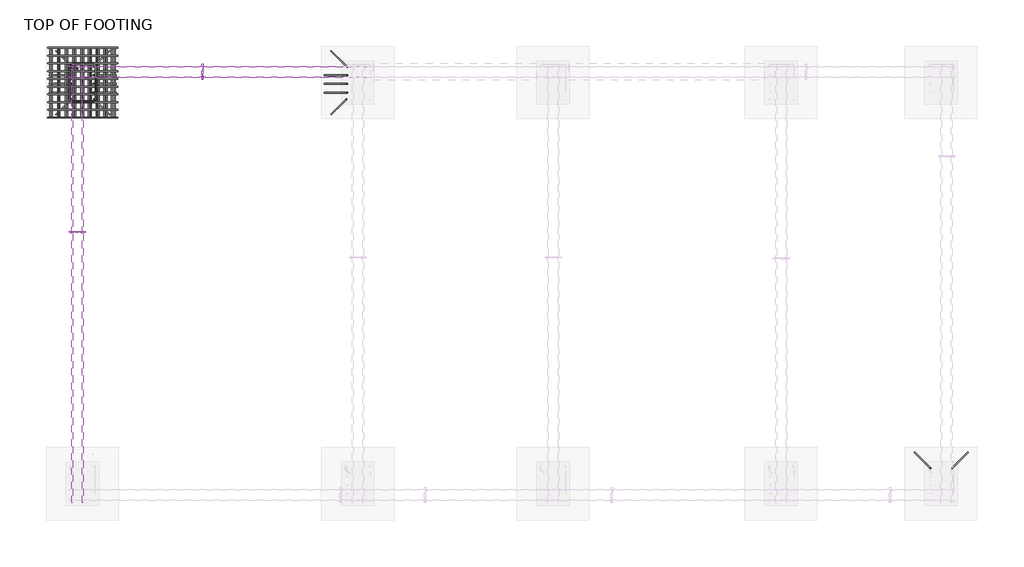
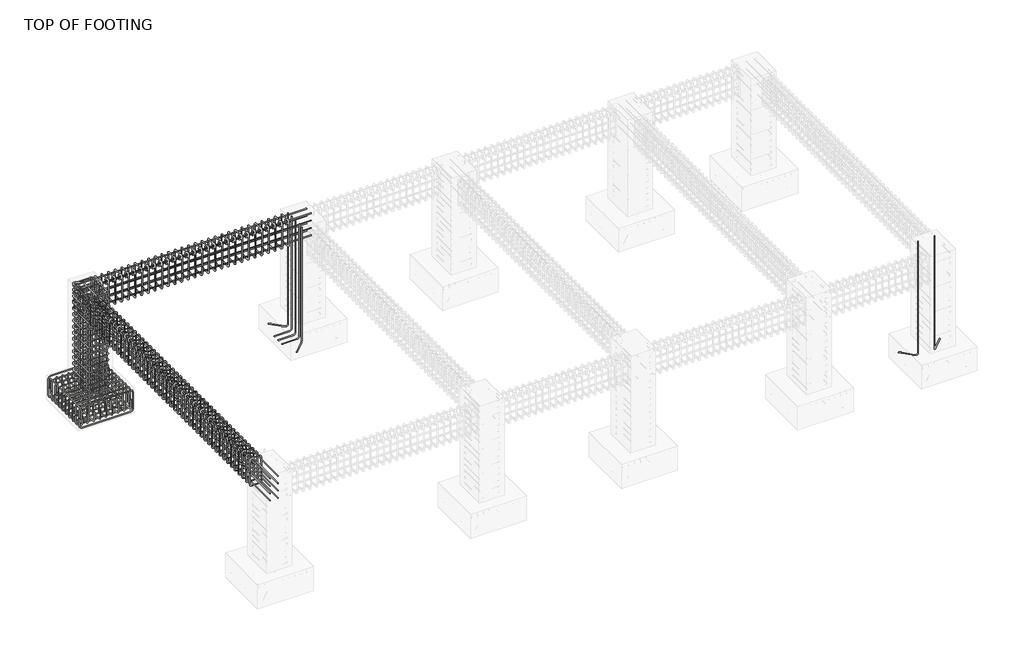
# One storey, part 5 of 9: 22 reinforcing bars.
"""IFC4 building model written with IfcOpenShell, lengths in millimetres."""

from ifc_helpers import new_model, si_unit, point, frame, origin, place, context, project, spatial, polyline, circle_curve, trimmed, segment, composite_curve, source, transform, mapped, element, save
from ifc_brep_helpers import swept_disk

model = new_model("IFC4")

# Units and contexts
model_context = context("Model", 3, world=origin())
ifc_project = project(units=[si_unit("LENGTHUNIT", "METRE", prefix="MILLI")], contexts=[model_context])

# Site, building, storey
site = spatial("IfcSite", under=ifc_project)
building = spatial("IfcBuilding", under=site)
storey = spatial("IfcBuildingStorey", under=building, Name="TOP OF FOOTING", Elevation=-1828.8)

# Reinforcing bars
placement = place(None, origin())
reinforcing_bar_shape = source(origin(), model_context, "Body", "SolidModel", [
    swept_disk(composite_curve([segment(polyline([(-11102.6174526, 4973.4875236, -2052.8356656), (-11102.6174526, 4973.4875236, -2200.1356656)]), True, "CONTINUOUS"), segment(trimmed(circle_curve(frame((-11148.9674526, 4973.4875236, -2200.1356656), z_axis=(0.0, 1.0, 0.0), x_axis=(46.350000000000364, 0.0, 0.0)), 46.35), [point((-11102.6174526, 4973.4875236, -2200.1356656))], [point((-11148.9674526, 4973.4875236, -2246.4856656))], True, "CARTESIAN"), True, "CONTINUOUS"), segment(polyline([(-11148.9674526, 4973.4875236, -2246.4856656), (-12017.5674526, 4973.4875236, -2246.4856656)]), True, "CONTINUOUS"), segment(trimmed(circle_curve(frame((-12017.5674526, 4973.4875236, -2200.1356656), z_axis=(0.0, 1.0, 0.0), x_axis=(0.0, 0.0, -46.350000000000364)), 46.35), [point((-12017.5674526, 4973.4875236, -2246.4856656))], [point((-12063.9174526, 4973.4875236, -2200.1356656))], True, "CARTESIAN"), True, "CONTINUOUS"), segment(polyline([(-12063.9174526, 4973.4875236, -2200.1356656), (-12063.9174526, 4973.4875236, -2052.8356656)]), True, "CONTINUOUS")], self_intersect=False), 6.35),
])
element("IfcReinforcingBar", 1, at=placement, inside=storey, context=model_context, shape_type="MappedRepresentation", body=[
    mapped(reinforcing_bar_shape, transform((0.0, 0.0, 0.0), x_axis=(1.0, 0.0, 0.0), y_axis=(0.0, 1.0, 0.0), z_axis=(0.0, 0.0, 1.0))),
    mapped(reinforcing_bar_shape, transform((0.0, -106.8111111, 0.0), x_axis=(1.0, 0.0, 0.0), y_axis=(0.0, 1.0, 0.0), z_axis=(0.0, 0.0, 1.0))),
    mapped(reinforcing_bar_shape, transform((0.0, -213.6222222, 0.0), x_axis=(1.0, 0.0, 0.0), y_axis=(0.0, 1.0, 0.0), z_axis=(0.0, 0.0, 1.0))),
    mapped(reinforcing_bar_shape, transform((0.0, -320.4333333, 0.0), x_axis=(1.0, 0.0, 0.0), y_axis=(0.0, 1.0, 0.0), z_axis=(0.0, 0.0, 1.0))),
    mapped(reinforcing_bar_shape, transform((0.0, -427.2444444, 0.0), x_axis=(1.0, 0.0, 0.0), y_axis=(0.0, 1.0, 0.0), z_axis=(0.0, 0.0, 1.0))),
    mapped(reinforcing_bar_shape, transform((0.0, -534.0555556, 0.0), x_axis=(1.0, 0.0, 0.0), y_axis=(0.0, 1.0, 0.0), z_axis=(0.0, 0.0, 1.0))),
    mapped(reinforcing_bar_shape, transform((0.0, -640.8666667, 0.0), x_axis=(1.0, 0.0, 0.0), y_axis=(0.0, 1.0, 0.0), z_axis=(0.0, 0.0, 1.0))),
    mapped(reinforcing_bar_shape, transform((0.0, -747.6777778, 0.0), x_axis=(1.0, 0.0, 0.0), y_axis=(0.0, 1.0, 0.0), z_axis=(0.0, 0.0, 1.0))),
    mapped(reinforcing_bar_shape, transform((0.0, -854.4888889, 0.0), x_axis=(1.0, 0.0, 0.0), y_axis=(0.0, 1.0, 0.0), z_axis=(0.0, 0.0, 1.0))),
    mapped(reinforcing_bar_shape, transform((0.0, -961.3, 0.0), x_axis=(1.0, 0.0, 0.0), y_axis=(0.0, 1.0, 0.0), z_axis=(0.0, 0.0, 1.0))),
])
reinforcing_bar_2_shape = source(origin(), model_context, "Body", "SolidModel", [
    swept_disk(composite_curve([segment(polyline([(-12063.9174526, 4973.4875236, -2041.8), (-12063.9174526, 4973.4875236, -1894.5)]), True, "CONTINUOUS"), segment(trimmed(circle_curve(frame((-12017.5674526, 4973.4875236, -1894.5), z_axis=(0.0, 1.0, 0.0), x_axis=(-46.350000000000364, 0.0, 0.0)), 46.35), [point((-12063.9174526, 4973.4875236, -1894.5))], [point((-12017.5674526, 4973.4875236, -1848.15))], True, "CARTESIAN"), True, "CONTINUOUS"), segment(polyline([(-12017.5674526, 4973.4875236, -1848.15), (-11148.9674526, 4973.4875236, -1848.15)]), True, "CONTINUOUS"), segment(trimmed(circle_curve(frame((-11148.9674526, 4973.4875236, -1894.5), z_axis=(0.0, 1.0, 0.0), x_axis=(0.0, 0.0, 46.34999999999991)), 46.35), [point((-11148.9674526, 4973.4875236, -1848.15))], [point((-11102.6174526, 4973.4875236, -1894.5))], True, "CARTESIAN"), True, "CONTINUOUS"), segment(polyline([(-11102.6174526, 4973.4875236, -1894.5), (-11102.6174526, 4973.4875236, -2041.8)]), True, "CONTINUOUS")], self_intersect=False), 6.35),
])
element("IfcReinforcingBar", 2, at=placement, inside=storey, context=model_context, shape_type="MappedRepresentation", body=[
    mapped(reinforcing_bar_2_shape, transform((0.0, 0.0, 0.0), x_axis=(1.0, 0.0, 0.0), y_axis=(0.0, 1.0, 0.0), z_axis=(0.0, 0.0, 1.0))),
    mapped(reinforcing_bar_2_shape, transform((0.0, -106.8111111, 0.0), x_axis=(1.0, 0.0, 0.0), y_axis=(0.0, 1.0, 0.0), z_axis=(0.0, 0.0, 1.0))),
    mapped(reinforcing_bar_2_shape, transform((0.0, -213.6222222, 0.0), x_axis=(1.0, 0.0, 0.0), y_axis=(0.0, 1.0, 0.0), z_axis=(0.0, 0.0, 1.0))),
    mapped(reinforcing_bar_2_shape, transform((0.0, -320.4333333, 0.0), x_axis=(1.0, 0.0, 0.0), y_axis=(0.0, 1.0, 0.0), z_axis=(0.0, 0.0, 1.0))),
    mapped(reinforcing_bar_2_shape, transform((0.0, -427.2444444, 0.0), x_axis=(1.0, 0.0, 0.0), y_axis=(0.0, 1.0, 0.0), z_axis=(0.0, 0.0, 1.0))),
    mapped(reinforcing_bar_2_shape, transform((0.0, -534.0555556, 0.0), x_axis=(1.0, 0.0, 0.0), y_axis=(0.0, 1.0, 0.0), z_axis=(0.0, 0.0, 1.0))),
    mapped(reinforcing_bar_2_shape, transform((0.0, -640.8666667, 0.0), x_axis=(1.0, 0.0, 0.0), y_axis=(0.0, 1.0, 0.0), z_axis=(0.0, 0.0, 1.0))),
    mapped(reinforcing_bar_2_shape, transform((0.0, -747.6777778, 0.0), x_axis=(1.0, 0.0, 0.0), y_axis=(0.0, 1.0, 0.0), z_axis=(0.0, 0.0, 1.0))),
    mapped(reinforcing_bar_2_shape, transform((0.0, -854.4888889, 0.0), x_axis=(1.0, 0.0, 0.0), y_axis=(0.0, 1.0, 0.0), z_axis=(0.0, 0.0, 1.0))),
    mapped(reinforcing_bar_2_shape, transform((0.0, -961.3, 0.0), x_axis=(1.0, 0.0, 0.0), y_axis=(0.0, 1.0, 0.0), z_axis=(0.0, 0.0, 1.0))),
])
reinforcing_bar_3_shape = source(origin(), model_context, "Body", "SolidModel", [
    swept_disk(composite_curve([segment(polyline([(-12013.2674526, 4973.4875236, -2020.15), (-12013.2674526, 4973.4875236, -2167.45)]), True, "CONTINUOUS"), segment(trimmed(circle_curve(frame((-12013.2674526, 4927.1375236, -2167.45), z_axis=(-1.0, 0.0, 0.0), x_axis=(0.0, 46.349999999999454, 0.0)), 46.35), [point((-12013.2674526, 4973.4875236, -2167.45))], [point((-12013.2674526, 4927.1375236, -2213.8))], True, "CARTESIAN"), True, "CONTINUOUS"), segment(polyline([(-12013.2674526, 4927.1375236, -2213.8), (-12013.2674526, 4058.5375236, -2213.8)]), True, "CONTINUOUS"), segment(trimmed(circle_curve(frame((-12013.2674526, 4058.5375236, -2167.45), z_axis=(-1.0, 0.0, 0.0), x_axis=(0.0, 0.0, -46.350000000000364)), 46.35), [point((-12013.2674526, 4058.5375236, -2213.8))], [point((-12013.2674526, 4012.1875236, -2167.45))], True, "CARTESIAN"), True, "CONTINUOUS"), segment(polyline([(-12013.2674526, 4012.1875236, -2167.45), (-12013.2674526, 4012.1875236, -2020.15)]), True, "CONTINUOUS")], self_intersect=False), 6.35),
])
element("IfcReinforcingBar", 3, at=placement, inside=storey, context=model_context, shape_type="MappedRepresentation", body=[
    mapped(reinforcing_bar_3_shape, transform((0.0, 0.0, 0.0), x_axis=(1.0, 0.0, 0.0), y_axis=(0.0, 1.0, 0.0), z_axis=(0.0, 0.0, 1.0))),
    mapped(reinforcing_bar_3_shape, transform((108.8370374, 0.0, 0.0), x_axis=(1.0, 0.0, 0.0), y_axis=(0.0, 1.0, 0.0), z_axis=(0.0, 0.0, 1.0))),
    mapped(reinforcing_bar_3_shape, transform((217.6740748, 0.0, 0.0), x_axis=(1.0, 0.0, 0.0), y_axis=(0.0, 1.0, 0.0), z_axis=(0.0, 0.0, 1.0))),
    mapped(reinforcing_bar_3_shape, transform((326.5111123, 0.0, 0.0), x_axis=(1.0, 0.0, 0.0), y_axis=(0.0, 1.0, 0.0), z_axis=(0.0, 0.0, 1.0))),
    mapped(reinforcing_bar_3_shape, transform((435.3481497, 0.0, 0.0), x_axis=(1.0, 0.0, 0.0), y_axis=(0.0, 1.0, 0.0), z_axis=(0.0, 0.0, 1.0))),
    mapped(reinforcing_bar_3_shape, transform((544.1851871, 0.0, 0.0), x_axis=(1.0, 0.0, 0.0), y_axis=(0.0, 1.0, 0.0), z_axis=(0.0, 0.0, 1.0))),
    mapped(reinforcing_bar_3_shape, transform((653.0222245, 0.0, 0.0), x_axis=(1.0, 0.0, 0.0), y_axis=(0.0, 1.0, 0.0), z_axis=(0.0, 0.0, 1.0))),
    mapped(reinforcing_bar_3_shape, transform((761.8592619, 0.0, 0.0), x_axis=(1.0, 0.0, 0.0), y_axis=(0.0, 1.0, 0.0), z_axis=(0.0, 0.0, 1.0))),
    mapped(reinforcing_bar_3_shape, transform((870.6962994, 0.0, 0.0), x_axis=(1.0, 0.0, 0.0), y_axis=(0.0, 1.0, 0.0), z_axis=(0.0, 0.0, 1.0))),
])
reinforcing_bar_4_shape = source(origin(), model_context, "Body", "SolidModel", [
    swept_disk(composite_curve([segment(polyline([(-11180.7455787, 4973.4875236, -2076.9782245), (-11180.7455787, 4973.4875236, -1929.6782245)]), True, "CONTINUOUS"), segment(trimmed(circle_curve(frame((-11180.7455787, 4927.1375236, -1929.6782245), z_axis=(1.0, 0.0, 0.0), x_axis=(0.0, 46.349999999999454, 0.0)), 46.35), [point((-11180.7455787, 4973.4875236, -1929.6782245))], [point((-11180.7455787, 4927.1375236, -1883.3282245))], True, "CARTESIAN"), True, "CONTINUOUS"), segment(polyline([(-11180.7455787, 4927.1375236, -1883.3282245), (-11180.7455787, 4058.5375236, -1883.3282245)]), True, "CONTINUOUS"), segment(trimmed(circle_curve(frame((-11180.7455787, 4058.5375236, -1929.6782245), z_axis=(1.0, 0.0, 0.0), x_axis=(0.0, 0.0, 46.34999999999991)), 46.35), [point((-11180.7455787, 4058.5375236, -1883.3282245))], [point((-11180.7455787, 4012.1875236, -1929.6782245))], True, "CARTESIAN"), True, "CONTINUOUS"), segment(polyline([(-11180.7455787, 4012.1875236, -1929.6782245), (-11180.7455787, 4012.1875236, -2076.9782245)]), True, "CONTINUOUS")], self_intersect=False), 6.35),
])
element("IfcReinforcingBar", 4, at=placement, inside=storey, context=model_context, shape_type="MappedRepresentation", body=[
    mapped(reinforcing_bar_4_shape, transform((0.0, 0.0, 0.0), x_axis=(1.0, 0.0, 0.0), y_axis=(0.0, 1.0, 0.0), z_axis=(0.0, 0.0, 1.0))),
    mapped(reinforcing_bar_4_shape, transform((-106.3275638, 0.0, 0.0), x_axis=(1.0, 0.0, 0.0), y_axis=(0.0, 1.0, 0.0), z_axis=(0.0, 0.0, 1.0))),
    mapped(reinforcing_bar_4_shape, transform((-212.6551275, 0.0, 0.0), x_axis=(1.0, 0.0, 0.0), y_axis=(0.0, 1.0, 0.0), z_axis=(0.0, 0.0, 1.0))),
    mapped(reinforcing_bar_4_shape, transform((-318.9826913, 0.0, 0.0), x_axis=(1.0, 0.0, 0.0), y_axis=(0.0, 1.0, 0.0), z_axis=(0.0, 0.0, 1.0))),
    mapped(reinforcing_bar_4_shape, transform((-425.310255, 0.0, 0.0), x_axis=(1.0, 0.0, 0.0), y_axis=(0.0, 1.0, 0.0), z_axis=(0.0, 0.0, 1.0))),
    mapped(reinforcing_bar_4_shape, transform((-531.6378188, 0.0, 0.0), x_axis=(1.0, 0.0, 0.0), y_axis=(0.0, 1.0, 0.0), z_axis=(0.0, 0.0, 1.0))),
    mapped(reinforcing_bar_4_shape, transform((-637.9653825, 0.0, 0.0), x_axis=(1.0, 0.0, 0.0), y_axis=(0.0, 1.0, 0.0), z_axis=(0.0, 0.0, 1.0))),
    mapped(reinforcing_bar_4_shape, transform((-744.2929463, 0.0, 0.0), x_axis=(1.0, 0.0, 0.0), y_axis=(0.0, 1.0, 0.0), z_axis=(0.0, 0.0, 1.0))),
    mapped(reinforcing_bar_4_shape, transform((-850.62051, 0.0, 0.0), x_axis=(1.0, 0.0, 0.0), y_axis=(0.0, 1.0, 0.0), z_axis=(0.0, 0.0, 1.0))),
])
reinforcing_bar_5_shape = source(origin(), model_context, "Body", "SolidModel", [
    swept_disk(composite_curve([segment(polyline([(-11730.5674526, 4357.3343029, -40.0), (-11730.5674526, 4357.3343029, -2148.1729582)]), True, "CONTINUOUS"), segment(trimmed(circle_curve(frame((-11776.9174526, 4357.3343029, -2148.1729582), z_axis=(0.0, 1.0, 0.0), x_axis=(46.350000000000364, 0.0, 0.0)), 46.35), [point((-11730.5674526, 4357.3343029, -2148.1729582))], [point((-11776.9174526, 4357.3343029, -2194.5229582))], True, "CARTESIAN"), True, "CONTINUOUS"), segment(polyline([(-11776.9174526, 4357.3343029, -2194.5229582), (-12043.513478, 4357.3343029, -2194.5229582)]), True, "CONTINUOUS")], self_intersect=False), 6.35),
])
element("IfcReinforcingBar", 5, at=placement, inside=storey, context=model_context, shape_type="MappedRepresentation", body=[
    mapped(reinforcing_bar_5_shape, transform((0.0, 0.0, 0.0), x_axis=(1.0, 0.0, 0.0), y_axis=(0.0, 1.0, 0.0), z_axis=(0.0, 0.0, 1.0))),
    mapped(reinforcing_bar_5_shape, transform((0.0, 119.1364467, 0.0), x_axis=(1.0, 0.0, 0.0), y_axis=(0.0, 1.0, 0.0), z_axis=(0.0, 0.0, 1.0))),
    mapped(reinforcing_bar_5_shape, transform((0.0, 238.2728934, 0.0), x_axis=(1.0, 0.0, 0.0), y_axis=(0.0, 1.0, 0.0), z_axis=(0.0, 0.0, 1.0))),
])
reinforcing_bar_6_shape = source(origin(), model_context, "Body", "SolidModel", [
    swept_disk(composite_curve([segment(polyline([(-11652.6560921, 4681.5617582, -1782.45), (-11708.399655, 4737.3053212, -1782.45)]), True, "CONTINUOUS"), segment(trimmed(circle_curve(frame((-11730.5674526, 4715.1375236, -1782.45), z_axis=(0.0, 0.0, 1.0), x_axis=(22.167797600000995, 22.167797600000085, 0.0)), 31.35), [point((-11708.399655, 4737.3053212, -1782.45))], [point((-11761.9174526, 4715.1375236, -1782.45))], True, "CARTESIAN"), True, "CONTINUOUS"), segment(polyline([(-11761.9174526, 4715.1375236, -1782.45), (-11761.9174526, 4270.5375236, -1782.45)]), True, "CONTINUOUS"), segment(trimmed(circle_curve(frame((-11730.5674526, 4270.5375236, -1782.45), z_axis=(0.0, 0.0, 1.0), x_axis=(-31.350000000000364, 0.0, 0.0)), 31.35), [point((-11761.9174526, 4270.5375236, -1782.45))], [point((-11730.5674526, 4239.1875236, -1782.45))], True, "CARTESIAN"), True, "CONTINUOUS"), segment(polyline([(-11730.5674526, 4239.1875236, -1782.45), (-11435.9674526, 4239.1875236, -1782.45)]), True, "CONTINUOUS"), segment(trimmed(circle_curve(frame((-11435.9674526, 4270.5277043, -1783.2345856), z_axis=(0.0, 0.025026655153786315, 0.9996867842138424), x_axis=(0.0, -31.34018070000002, 0.7845855999999003)), 31.35), [point((-11435.9674526, 4239.1875236, -1782.45))], [point((-11404.6174526, 4270.5277043, -1783.2345856))], True, "CARTESIAN"), True, "CONTINUOUS"), segment(polyline([(-11404.6174526, 4270.5277043, -1783.2345856), (-11404.6174526, 4715.1473429, -1794.3654144)]), True, "CONTINUOUS"), segment(trimmed(circle_curve(frame((-11435.9674526, 4715.1473429, -1794.3654144), z_axis=(0.0, 0.025026655153786315, 0.9996867842138424), x_axis=(31.350000000000364, 0.0, 0.0)), 31.35), [point((-11404.6174526, 4715.1473429, -1794.3654144))], [point((-11435.9674526, 4746.4875236, -1795.15))], True, "CARTESIAN"), True, "CONTINUOUS"), segment(polyline([(-11435.9674526, 4746.4875236, -1795.15), (-11730.5674526, 4746.4875236, -1795.15)]), True, "CONTINUOUS"), segment(trimmed(circle_curve(frame((-11730.5674526, 4715.1375236, -1795.15), z_axis=(0.0, 0.0, 1.0), x_axis=(0.0, 31.349999999999454, 0.0)), 31.35), [point((-11730.5674526, 4746.4875236, -1795.15))], [point((-11752.7352502, 4692.969726, -1795.15))], True, "CARTESIAN"), True, "CONTINUOUS"), segment(polyline([(-11752.7352502, 4692.969726, -1795.15), (-11696.9916873, 4637.226163, -1795.15)]), True, "CONTINUOUS")], self_intersect=False), 6.35),
])
element("IfcReinforcingBar", 6, at=placement, inside=storey, context=model_context, shape_type="MappedRepresentation", body=[
    mapped(reinforcing_bar_6_shape, transform((0.0, 0.0, 0.0), x_axis=(1.0, 0.0, 0.0), y_axis=(0.0, 1.0, 0.0), z_axis=(0.0, 0.0, 1.0))),
    mapped(reinforcing_bar_6_shape, transform((0.0, 0.0, 115.74), x_axis=(1.0, 0.0, 0.0), y_axis=(0.0, 1.0, 0.0), z_axis=(0.0, 0.0, 1.0))),
    mapped(reinforcing_bar_6_shape, transform((0.0, 0.0, 231.48), x_axis=(1.0, 0.0, 0.0), y_axis=(0.0, 1.0, 0.0), z_axis=(0.0, 0.0, 1.0))),
    mapped(reinforcing_bar_6_shape, transform((0.0, 0.0, 347.22), x_axis=(1.0, 0.0, 0.0), y_axis=(0.0, 1.0, 0.0), z_axis=(0.0, 0.0, 1.0))),
    mapped(reinforcing_bar_6_shape, transform((0.0, 0.0, 462.96), x_axis=(1.0, 0.0, 0.0), y_axis=(0.0, 1.0, 0.0), z_axis=(0.0, 0.0, 1.0))),
    mapped(reinforcing_bar_6_shape, transform((0.0, 0.0, 578.7), x_axis=(1.0, 0.0, 0.0), y_axis=(0.0, 1.0, 0.0), z_axis=(0.0, 0.0, 1.0))),
    mapped(reinforcing_bar_6_shape, transform((0.0, 0.0, 694.44), x_axis=(1.0, 0.0, 0.0), y_axis=(0.0, 1.0, 0.0), z_axis=(0.0, 0.0, 1.0))),
    mapped(reinforcing_bar_6_shape, transform((0.0, 0.0, 810.18), x_axis=(1.0, 0.0, 0.0), y_axis=(0.0, 1.0, 0.0), z_axis=(0.0, 0.0, 1.0))),
    mapped(reinforcing_bar_6_shape, transform((0.0, 0.0, 925.92), x_axis=(1.0, 0.0, 0.0), y_axis=(0.0, 1.0, 0.0), z_axis=(0.0, 0.0, 1.0))),
    mapped(reinforcing_bar_6_shape, transform((0.0, 0.0, 1041.66), x_axis=(1.0, 0.0, 0.0), y_axis=(0.0, 1.0, 0.0), z_axis=(0.0, 0.0, 1.0))),
    mapped(reinforcing_bar_6_shape, transform((0.0, 0.0, 1157.4), x_axis=(1.0, 0.0, 0.0), y_axis=(0.0, 1.0, 0.0), z_axis=(0.0, 0.0, 1.0))),
    mapped(reinforcing_bar_6_shape, transform((0.0, 0.0, 1273.14), x_axis=(1.0, 0.0, 0.0), y_axis=(0.0, 1.0, 0.0), z_axis=(0.0, 0.0, 1.0))),
    mapped(reinforcing_bar_6_shape, transform((0.0, 0.0, 1388.88), x_axis=(1.0, 0.0, 0.0), y_axis=(0.0, 1.0, 0.0), z_axis=(0.0, 0.0, 1.0))),
    mapped(reinforcing_bar_6_shape, transform((0.0, 0.0, 1504.62), x_axis=(1.0, 0.0, 0.0), y_axis=(0.0, 1.0, 0.0), z_axis=(0.0, 0.0, 1.0))),
    mapped(reinforcing_bar_6_shape, transform((0.0, 0.0, 1620.36), x_axis=(1.0, 0.0, 0.0), y_axis=(0.0, 1.0, 0.0), z_axis=(0.0, 0.0, 1.0))),
    mapped(reinforcing_bar_6_shape, transform((0.0, 0.0, 1736.1), x_axis=(1.0, 0.0, 0.0), y_axis=(0.0, 1.0, 0.0), z_axis=(0.0, 0.0, 1.0))),
])
element("IfcReinforcingBar", 7, at=placement, inside=storey, context=model_context, shape_type="SolidModel", body=[
    swept_disk(composite_curve([segment(polyline([(-11730.5674526, 4712.2713987, -40.0), (-11730.5674526, 4712.2713987, -2148.1729582)]), True, "CONTINUOUS"), segment(trimmed(circle_curve(frame((-11763.3418519, 4745.045798, -2148.1729582), z_axis=(0.7071067811865507, 0.7071067811865444, 0.0), x_axis=(32.77439930000037, -32.77439930000037, 0.0)), 46.35), [point((-11730.5674526, 4712.2713987, -2148.1729582))], [point((-11763.3418519, 4745.045798, -2194.5229582))], True, "CARTESIAN"), True, "CONTINUOUS"), segment(polyline([(-11763.3418519, 4745.045798, -2194.5229582), (-11951.8537093, 4933.5576554, -2194.5229582)]), True, "CONTINUOUS")], self_intersect=False), 6.35),
])
element("IfcReinforcingBar", 8, at=placement, inside=storey, context=model_context, shape_type="SolidModel", body=[
    swept_disk(composite_curve([segment(polyline([(-11740.5132324, 4263.4578687, -40.0), (-11740.5132324, 4263.4578687, -2148.1729582)]), True, "CONTINUOUS"), segment(trimmed(circle_curve(frame((-11773.2876317, 4230.6834694, -2148.1729582), z_axis=(-0.707106781186547, 0.707106781186548, 0.0), x_axis=(32.77439929999855, 32.77439930000037, 0.0)), 46.35), [point((-11740.5132324, 4263.4578687, -2148.1729582))], [point((-11773.2876317, 4230.6834694, -2194.5229582))], True, "CARTESIAN"), True, "CONTINUOUS"), segment(polyline([(-11773.2876317, 4230.6834694, -2194.5229582), (-11951.8537093, 4052.1173918, -2194.5229582)]), True, "CONTINUOUS")], self_intersect=False), 6.35),
])
element("IfcReinforcingBar", 9, at=placement, inside=storey, context=model_context, shape_type="SolidModel", body=[
    swept_disk(composite_curve([segment(polyline([(-11435.9674526, 4712.2713987, -40.0), (-11435.9674526, 4712.2713987, -2148.1729582)]), True, "CONTINUOUS"), segment(trimmed(circle_curve(frame((-11403.1930533, 4745.045798, -2148.1729582), z_axis=(0.7071067811865507, -0.7071067811865444, 0.0), x_axis=(-32.77439930000037, -32.77439930000037, 0.0)), 46.35), [point((-11435.9674526, 4712.2713987, -2148.1729582))], [point((-11403.1930533, 4745.045798, -2194.5229582))], True, "CARTESIAN"), True, "CONTINUOUS"), segment(polyline([(-11403.1930533, 4745.045798, -2194.5229582), (-11214.6811959, 4933.5576554, -2194.5229582)]), True, "CONTINUOUS")], self_intersect=False), 6.35),
])
element("IfcReinforcingBar", 10, at=placement, inside=storey, context=model_context, shape_type="SolidModel", body=[
    swept_disk(composite_curve([segment(polyline([(-11426.0216728, 4263.4578687, -40.0), (-11426.0216728, 4263.4578687, -2148.1729582)]), True, "CONTINUOUS"), segment(trimmed(circle_curve(frame((-11393.2472735, 4230.6834694, -2148.1729582), z_axis=(-0.707106781186547, -0.707106781186548, 0.0), x_axis=(-32.77439930000037, 32.77439930000037, 0.0)), 46.35), [point((-11426.0216728, 4263.4578687, -2148.1729582))], [point((-11393.2472735, 4230.6834694, -2194.5229582))], True, "CARTESIAN"), True, "CONTINUOUS"), segment(polyline([(-11393.2472735, 4230.6834694, -2194.5229582), (-11214.6811959, 4052.1173918, -2194.5229582)]), True, "CONTINUOUS")], self_intersect=False), 6.35),
])
reinforcing_bar_7_shape = source(origin(), model_context, "Body", "SolidModel", [
    swept_disk(composite_curve([segment(polyline([(-11435.9674526, 4357.3343029, -40.0), (-11435.9674526, 4357.3343029, -2148.1729582)]), True, "CONTINUOUS"), segment(trimmed(circle_curve(frame((-11389.6174526, 4357.3343029, -2148.1729582), z_axis=(0.0, -1.0, 0.0), x_axis=(-46.350000000000364, 0.0, 0.0)), 46.35), [point((-11435.9674526, 4357.3343029, -2148.1729582))], [point((-11389.6174526, 4357.3343029, -2194.5229582))], True, "CARTESIAN"), True, "CONTINUOUS"), segment(polyline([(-11389.6174526, 4357.3343029, -2194.5229582), (-11123.0214272, 4357.3343029, -2194.5229582)]), True, "CONTINUOUS")], self_intersect=False), 6.35),
])
element("IfcReinforcingBar", 11, at=placement, inside=storey, context=model_context, shape_type="MappedRepresentation", body=[
    mapped(reinforcing_bar_7_shape, transform((0.0, 0.0, 0.0), x_axis=(1.0, 0.0, 0.0), y_axis=(0.0, 1.0, 0.0), z_axis=(0.0, 0.0, 1.0))),
    mapped(reinforcing_bar_7_shape, transform((0.0, 119.1364467, 0.0), x_axis=(1.0, 0.0, 0.0), y_axis=(0.0, 1.0, 0.0), z_axis=(0.0, 0.0, 1.0))),
    mapped(reinforcing_bar_7_shape, transform((0.0, 238.2728934, 0.0), x_axis=(1.0, 0.0, 0.0), y_axis=(0.0, 1.0, 0.0), z_axis=(0.0, 0.0, 1.0))),
])
reinforcing_bar_8_shape = source(origin(), model_context, "Body", "SolidModel", [
    swept_disk(composite_curve([segment(polyline([(-7930.5674526, 4357.3343029, -40.0), (-7930.5674526, 4357.3343029, -2148.1729582)]), True, "CONTINUOUS"), segment(trimmed(circle_curve(frame((-7976.9174526, 4357.3343029, -2148.1729582), z_axis=(0.0, 1.0, 0.0), x_axis=(46.349999999999454, 0.0, 0.0)), 46.35), [point((-7930.5674526, 4357.3343029, -2148.1729582))], [point((-7976.9174526, 4357.3343029, -2194.5229582))], True, "CARTESIAN"), True, "CONTINUOUS"), segment(polyline([(-7976.9174526, 4357.3343029, -2194.5229582), (-8243.513478, 4357.3343029, -2194.5229582)]), True, "CONTINUOUS")], self_intersect=False), 6.35),
])
element("IfcReinforcingBar", 12, at=placement, inside=storey, context=model_context, shape_type="MappedRepresentation", body=[
    mapped(reinforcing_bar_8_shape, transform((0.0, 0.0, 0.0), x_axis=(1.0, 0.0, 0.0), y_axis=(0.0, 1.0, 0.0), z_axis=(0.0, 0.0, 1.0))),
    mapped(reinforcing_bar_8_shape, transform((0.0, 119.1364467, 0.0), x_axis=(1.0, 0.0, 0.0), y_axis=(0.0, 1.0, 0.0), z_axis=(0.0, 0.0, 1.0))),
    mapped(reinforcing_bar_8_shape, transform((0.0, 238.2728934, 0.0), x_axis=(1.0, 0.0, 0.0), y_axis=(0.0, 1.0, 0.0), z_axis=(0.0, 0.0, 1.0))),
])
element("IfcReinforcingBar", 13, at=placement, inside=storey, context=model_context, shape_type="SolidModel", body=[
    swept_disk(composite_curve([segment(polyline([(-7930.5674526, 4712.2713987, -40.0), (-7930.5674526, 4712.2713987, -2148.1729582)]), True, "CONTINUOUS"), segment(trimmed(circle_curve(frame((-7963.3418519, 4745.045798, -2148.1729582), z_axis=(0.7071067811865507, 0.7071067811865444, 0.0), x_axis=(32.77439929999946, -32.77439930000037, 0.0)), 46.35), [point((-7930.5674526, 4712.2713987, -2148.1729582))], [point((-7963.3418519, 4745.045798, -2194.5229582))], True, "CARTESIAN"), True, "CONTINUOUS"), segment(polyline([(-7963.3418519, 4745.045798, -2194.5229582), (-8151.8537093, 4933.5576554, -2194.5229582)]), True, "CONTINUOUS")], self_intersect=False), 6.35),
])
element("IfcReinforcingBar", 14, at=placement, inside=storey, context=model_context, shape_type="SolidModel", body=[
    swept_disk(composite_curve([segment(polyline([(-7940.5132324, 4263.4578687, -40.0), (-7940.5132324, 4263.4578687, -2148.1729582)]), True, "CONTINUOUS"), segment(trimmed(circle_curve(frame((-7973.2876317, 4230.6834694, -2148.1729582), z_axis=(-0.707106781186547, 0.707106781186548, 0.0), x_axis=(32.77439930000037, 32.77439930000037, 0.0)), 46.35), [point((-7940.5132324, 4263.4578687, -2148.1729582))], [point((-7973.2876317, 4230.6834694, -2194.5229582))], True, "CARTESIAN"), True, "CONTINUOUS"), segment(polyline([(-7973.2876317, 4230.6834694, -2194.5229582), (-8151.8537093, 4052.1173918, -2194.5229582)]), True, "CONTINUOUS")], self_intersect=False), 6.35),
])
element("IfcReinforcingBar", 15, at=placement, inside=storey, context=model_context, shape_type="SolidModel", body=[
    swept_disk(composite_curve([segment(polyline([(129.4325474, -832.8986176, -40.0), (129.4325474, -832.8986176, -2148.1729582)]), True, "CONTINUOUS"), segment(trimmed(circle_curve(frame((96.6581481, -800.1242183, -2148.1729582), z_axis=(0.7071067811865507, 0.7071067811865444, 0.0), x_axis=(32.7743993, -32.774399299999914, 0.0)), 46.35), [point((129.4325474, -832.8986176, -2148.1729582))], [point((96.6581481, -800.1242183, -2194.5229582))], True, "CARTESIAN"), True, "CONTINUOUS"), segment(polyline([(96.6581481, -800.1242183, -2194.5229582), (-91.8537093, -611.6123609, -2194.5229582)]), True, "CONTINUOUS")], self_intersect=False), 6.35),
])
element("IfcReinforcingBar", 16, at=placement, inside=storey, context=model_context, shape_type="SolidModel", body=[
    swept_disk(composite_curve([segment(polyline([(424.0325474, -832.8986176, -40.0), (424.0325474, -832.8986176, -2148.1729582)]), True, "CONTINUOUS"), segment(trimmed(circle_curve(frame((456.8069467, -800.1242183, -2148.1729582), z_axis=(0.7071067811865507, -0.7071067811865444, 0.0), x_axis=(-32.77439930000003, -32.774399299999914, 0.0)), 46.35), [point((424.0325474, -832.8986176, -2148.1729582))], [point((456.8069467, -800.1242183, -2194.5229582))], True, "CARTESIAN"), True, "CONTINUOUS"), segment(polyline([(456.8069467, -800.1242183, -2194.5229582), (645.3188041, -611.6123609, -2194.5229582)]), True, "CONTINUOUS")], self_intersect=False), 6.35),
])
reinforcing_bar_9_shape = source(origin(), model_context, "Body", "SolidModel", [
    swept_disk(composite_curve([segment(polyline([(-11652.6560921, 4186.4875236, -111.2757654), (-11708.399655, 4186.4875236, -55.5322024)]), True, "CONTINUOUS"), segment(trimmed(circle_curve(frame((-11730.5674526, 4186.4875236, -77.7), z_axis=(0.0, -1.0, 0.0), x_axis=(22.167797600000995, 0.0, 22.1677976)), 31.35), [point((-11708.399655, 4186.4875236, -55.5322024))], [point((-11761.9174526, 4186.4875236, -77.7))], True, "CARTESIAN"), True, "CONTINUOUS"), segment(polyline([(-11761.9174526, 4186.4875236, -77.7), (-11761.9174526, 4186.4875236, -522.3)]), True, "CONTINUOUS"), segment(trimmed(circle_curve(frame((-11730.5674526, 4186.4875236, -522.3), z_axis=(0.0, -1.0, 0.0), x_axis=(-31.350000000000364, 0.0, 0.0)), 31.35), [point((-11761.9174526, 4186.4875236, -522.3))], [point((-11730.5674526, 4186.4875236, -553.65))], True, "CARTESIAN"), True, "CONTINUOUS"), segment(polyline([(-11730.5674526, 4186.4875236, -553.65), (-11585.9674526, 4186.4875236, -553.65)]), True, "CONTINUOUS"), segment(trimmed(circle_curve(frame((-11585.9674526, 4187.2721092, -522.3098193), z_axis=(0.0, -0.9996867842138424, 0.025026655153786322), x_axis=(0.0, -0.784585600000355, -31.34018070000002)), 31.35), [point((-11585.9674526, 4186.4875236, -553.65))], [point((-11554.6174526, 4187.2721092, -522.3098193))], True, "CARTESIAN"), True, "CONTINUOUS"), segment(polyline([(-11554.6174526, 4187.2721092, -522.3098193), (-11554.6174526, 4198.4029379, -77.6901807)]), True, "CONTINUOUS"), segment(trimmed(circle_curve(frame((-11585.9674526, 4198.4029379, -77.6901807), z_axis=(0.0, -0.9996867842138424, 0.025026655153786322), x_axis=(31.350000000000364, 0.0, 0.0)), 31.35), [point((-11554.6174526, 4198.4029379, -77.6901807))], [point((-11585.9674526, 4199.1875236, -46.35))], True, "CARTESIAN"), True, "CONTINUOUS"), segment(polyline([(-11585.9674526, 4199.1875236, -46.35), (-11730.5674526, 4199.1875236, -46.35)]), True, "CONTINUOUS"), segment(trimmed(circle_curve(frame((-11730.5674526, 4199.1875236, -77.7), z_axis=(0.0, -1.0, 0.0), x_axis=(0.0, 0.0, 31.35)), 31.35), [point((-11730.5674526, 4199.1875236, -46.35))], [point((-11752.7352502, 4199.1875236, -99.8677976))], True, "CARTESIAN"), True, "CONTINUOUS"), segment(polyline([(-11752.7352502, 4199.1875236, -99.8677976), (-11696.9916873, 4199.1875236, -155.6113605)]), True, "CONTINUOUS")], self_intersect=False), 6.35),
])
element("IfcReinforcingBar", 17, at=placement, inside=storey, context=model_context, shape_type="MappedRepresentation", body=[
    mapped(reinforcing_bar_9_shape, transform((0.0, 0.0, 0.0), x_axis=(1.0, 0.0, 0.0), y_axis=(0.0, 1.0, 0.0), z_axis=(0.0, 0.0, 1.0))),
    mapped(reinforcing_bar_9_shape, transform((0.0, -117.4397623, 0.0), x_axis=(1.0, 0.0, 0.0), y_axis=(0.0, 1.0, 0.0), z_axis=(0.0, 0.0, 1.0))),
    mapped(reinforcing_bar_9_shape, transform((0.0, -234.8795246, 0.0), x_axis=(1.0, 0.0, 0.0), y_axis=(0.0, 1.0, 0.0), z_axis=(0.0, 0.0, 1.0))),
    mapped(reinforcing_bar_9_shape, transform((0.0, -352.3192869, 0.0), x_axis=(1.0, 0.0, 0.0), y_axis=(0.0, 1.0, 0.0), z_axis=(0.0, 0.0, 1.0))),
    mapped(reinforcing_bar_9_shape, transform((0.0, -469.7590492, 0.0), x_axis=(1.0, 0.0, 0.0), y_axis=(0.0, 1.0, 0.0), z_axis=(0.0, 0.0, 1.0))),
    mapped(reinforcing_bar_9_shape, transform((0.0, -587.1988115, 0.0), x_axis=(1.0, 0.0, 0.0), y_axis=(0.0, 1.0, 0.0), z_axis=(0.0, 0.0, 1.0))),
    mapped(reinforcing_bar_9_shape, transform((0.0, -704.6385738, 0.0), x_axis=(1.0, 0.0, 0.0), y_axis=(0.0, 1.0, 0.0), z_axis=(0.0, 0.0, 1.0))),
    mapped(reinforcing_bar_9_shape, transform((0.0, -822.0783361, 0.0), x_axis=(1.0, 0.0, 0.0), y_axis=(0.0, 1.0, 0.0), z_axis=(0.0, 0.0, 1.0))),
    mapped(reinforcing_bar_9_shape, transform((0.0, -939.5180983, 0.0), x_axis=(1.0, 0.0, 0.0), y_axis=(0.0, 1.0, 0.0), z_axis=(0.0, 0.0, 1.0))),
    mapped(reinforcing_bar_9_shape, transform((0.0, -1056.9578606, 0.0), x_axis=(1.0, 0.0, 0.0), y_axis=(0.0, 1.0, 0.0), z_axis=(0.0, 0.0, 1.0))),
    mapped(reinforcing_bar_9_shape, transform((0.0, -1174.3976229, 0.0), x_axis=(1.0, 0.0, 0.0), y_axis=(0.0, 1.0, 0.0), z_axis=(0.0, 0.0, 1.0))),
    mapped(reinforcing_bar_9_shape, transform((0.0, -1291.8373852, 0.0), x_axis=(1.0, 0.0, 0.0), y_axis=(0.0, 1.0, 0.0), z_axis=(0.0, 0.0, 1.0))),
    mapped(reinforcing_bar_9_shape, transform((0.0, -1409.2771475, 0.0), x_axis=(1.0, 0.0, 0.0), y_axis=(0.0, 1.0, 0.0), z_axis=(0.0, 0.0, 1.0))),
    mapped(reinforcing_bar_9_shape, transform((0.0, -1526.7169098, 0.0), x_axis=(1.0, 0.0, 0.0), y_axis=(0.0, 1.0, 0.0), z_axis=(0.0, 0.0, 1.0))),
    mapped(reinforcing_bar_9_shape, transform((0.0, -1644.1566721, 0.0), x_axis=(1.0, 0.0, 0.0), y_axis=(0.0, 1.0, 0.0), z_axis=(0.0, 0.0, 1.0))),
    mapped(reinforcing_bar_9_shape, transform((0.0, -1761.5964344, 0.0), x_axis=(1.0, 0.0, 0.0), y_axis=(0.0, 1.0, 0.0), z_axis=(0.0, 0.0, 1.0))),
    mapped(reinforcing_bar_9_shape, transform((0.0, -1879.0361967, 0.0), x_axis=(1.0, 0.0, 0.0), y_axis=(0.0, 1.0, 0.0), z_axis=(0.0, 0.0, 1.0))),
    mapped(reinforcing_bar_9_shape, transform((0.0, -1996.475959, 0.0), x_axis=(1.0, 0.0, 0.0), y_axis=(0.0, 1.0, 0.0), z_axis=(0.0, 0.0, 1.0))),
    mapped(reinforcing_bar_9_shape, transform((0.0, -2113.9157213, 0.0), x_axis=(1.0, 0.0, 0.0), y_axis=(0.0, 1.0, 0.0), z_axis=(0.0, 0.0, 1.0))),
    mapped(reinforcing_bar_9_shape, transform((0.0, -2231.3554836, 0.0), x_axis=(1.0, 0.0, 0.0), y_axis=(0.0, 1.0, 0.0), z_axis=(0.0, 0.0, 1.0))),
    mapped(reinforcing_bar_9_shape, transform((0.0, -2348.7952459, 0.0), x_axis=(1.0, 0.0, 0.0), y_axis=(0.0, 1.0, 0.0), z_axis=(0.0, 0.0, 1.0))),
    mapped(reinforcing_bar_9_shape, transform((0.0, -2466.2350082, 0.0), x_axis=(1.0, 0.0, 0.0), y_axis=(0.0, 1.0, 0.0), z_axis=(0.0, 0.0, 1.0))),
    mapped(reinforcing_bar_9_shape, transform((0.0, -2583.6747705, 0.0), x_axis=(1.0, 0.0, 0.0), y_axis=(0.0, 1.0, 0.0), z_axis=(0.0, 0.0, 1.0))),
    mapped(reinforcing_bar_9_shape, transform((0.0, -2701.1145327, 0.0), x_axis=(1.0, 0.0, 0.0), y_axis=(0.0, 1.0, 0.0), z_axis=(0.0, 0.0, 1.0))),
    mapped(reinforcing_bar_9_shape, transform((0.0, -2818.554295, 0.0), x_axis=(1.0, 0.0, 0.0), y_axis=(0.0, 1.0, 0.0), z_axis=(0.0, 0.0, 1.0))),
    mapped(reinforcing_bar_9_shape, transform((0.0, -2935.9940573, 0.0), x_axis=(1.0, 0.0, 0.0), y_axis=(0.0, 1.0, 0.0), z_axis=(0.0, 0.0, 1.0))),
    mapped(reinforcing_bar_9_shape, transform((0.0, -3053.4338196, 0.0), x_axis=(1.0, 0.0, 0.0), y_axis=(0.0, 1.0, 0.0), z_axis=(0.0, 0.0, 1.0))),
    mapped(reinforcing_bar_9_shape, transform((0.0, -3170.8735819, 0.0), x_axis=(1.0, 0.0, 0.0), y_axis=(0.0, 1.0, 0.0), z_axis=(0.0, 0.0, 1.0))),
    mapped(reinforcing_bar_9_shape, transform((0.0, -3288.3133442, 0.0), x_axis=(1.0, 0.0, 0.0), y_axis=(0.0, 1.0, 0.0), z_axis=(0.0, 0.0, 1.0))),
    mapped(reinforcing_bar_9_shape, transform((0.0, -3405.7531065, 0.0), x_axis=(1.0, 0.0, 0.0), y_axis=(0.0, 1.0, 0.0), z_axis=(0.0, 0.0, 1.0))),
    mapped(reinforcing_bar_9_shape, transform((0.0, -3523.1928688, 0.0), x_axis=(1.0, 0.0, 0.0), y_axis=(0.0, 1.0, 0.0), z_axis=(0.0, 0.0, 1.0))),
    mapped(reinforcing_bar_9_shape, transform((0.0, -3640.6326311, 0.0), x_axis=(1.0, 0.0, 0.0), y_axis=(0.0, 1.0, 0.0), z_axis=(0.0, 0.0, 1.0))),
    mapped(reinforcing_bar_9_shape, transform((0.0, -3758.0723934, 0.0), x_axis=(1.0, 0.0, 0.0), y_axis=(0.0, 1.0, 0.0), z_axis=(0.0, 0.0, 1.0))),
    mapped(reinforcing_bar_9_shape, transform((0.0, -3875.5121557, 0.0), x_axis=(1.0, 0.0, 0.0), y_axis=(0.0, 1.0, 0.0), z_axis=(0.0, 0.0, 1.0))),
    mapped(reinforcing_bar_9_shape, transform((0.0, -3992.951918, 0.0), x_axis=(1.0, 0.0, 0.0), y_axis=(0.0, 1.0, 0.0), z_axis=(0.0, 0.0, 1.0))),
    mapped(reinforcing_bar_9_shape, transform((0.0, -4110.3916803, 0.0), x_axis=(1.0, 0.0, 0.0), y_axis=(0.0, 1.0, 0.0), z_axis=(0.0, 0.0, 1.0))),
    mapped(reinforcing_bar_9_shape, transform((0.0, -4227.8314426, 0.0), x_axis=(1.0, 0.0, 0.0), y_axis=(0.0, 1.0, 0.0), z_axis=(0.0, 0.0, 1.0))),
    mapped(reinforcing_bar_9_shape, transform((0.0, -4345.2712048, 0.0), x_axis=(1.0, 0.0, 0.0), y_axis=(0.0, 1.0, 0.0), z_axis=(0.0, 0.0, 1.0))),
    mapped(reinforcing_bar_9_shape, transform((0.0, -4462.7109671, 0.0), x_axis=(1.0, 0.0, 0.0), y_axis=(0.0, 1.0, 0.0), z_axis=(0.0, 0.0, 1.0))),
    mapped(reinforcing_bar_9_shape, transform((0.0, -4580.1507294, 0.0), x_axis=(1.0, 0.0, 0.0), y_axis=(0.0, 1.0, 0.0), z_axis=(0.0, 0.0, 1.0))),
    mapped(reinforcing_bar_9_shape, transform((0.0, -4697.5904917, 0.0), x_axis=(1.0, 0.0, 0.0), y_axis=(0.0, 1.0, 0.0), z_axis=(0.0, 0.0, 1.0))),
    mapped(reinforcing_bar_9_shape, transform((0.0, -4815.030254, 0.0), x_axis=(1.0, 0.0, 0.0), y_axis=(0.0, 1.0, 0.0), z_axis=(0.0, 0.0, 1.0))),
    mapped(reinforcing_bar_9_shape, transform((0.0, -4932.4700163, 0.0), x_axis=(1.0, 0.0, 0.0), y_axis=(0.0, 1.0, 0.0), z_axis=(0.0, 0.0, 1.0))),
])
reinforcing_bar_10_shape = source(origin(), model_context, "Body", "SolidModel", [
    swept_disk(composite_curve([segment(polyline([(-11730.5674526, 4752.8375236, -80.0), (-11730.5674526, -1312.3324927, -80.0)]), True, "CONTINUOUS")], self_intersect=False), 6.35),
])
element("IfcReinforcingBar", 18, at=placement, inside=storey, context=model_context, shape_type="MappedRepresentation", body=[
    mapped(reinforcing_bar_10_shape, transform((0.0, 0.0, 0.0), x_axis=(1.0, 0.0, 0.0), y_axis=(0.0, 1.0, 0.0), z_axis=(0.0, 0.0, 1.0))),
    mapped(reinforcing_bar_10_shape, transform((0.0, 0.0, -138.5031468), x_axis=(1.0, 0.0, 0.0), y_axis=(0.0, 1.0, 0.0), z_axis=(0.0, 0.0, 1.0))),
    mapped(reinforcing_bar_10_shape, transform((0.0, 0.0, -277.0062937), x_axis=(1.0, 0.0, 0.0), y_axis=(0.0, 1.0, 0.0), z_axis=(0.0, 0.0, 1.0))),
    mapped(reinforcing_bar_10_shape, transform((0.0, 0.0, -415.5094405), x_axis=(1.0, 0.0, 0.0), y_axis=(0.0, 1.0, 0.0), z_axis=(0.0, 0.0, 1.0))),
])
reinforcing_bar_11_shape = source(origin(), model_context, "Body", "SolidModel", [
    swept_disk(composite_curve([segment(polyline([(-11585.9674526, 4752.8375236, -80.0), (-11585.9674526, -1312.3324927, -80.0)]), True, "CONTINUOUS")], self_intersect=False), 6.35),
])
element("IfcReinforcingBar", 19, at=placement, inside=storey, context=model_context, shape_type="MappedRepresentation", body=[
    mapped(reinforcing_bar_11_shape, transform((0.0, 0.0, 0.0), x_axis=(1.0, 0.0, 0.0), y_axis=(0.0, 1.0, 0.0), z_axis=(0.0, 0.0, 1.0))),
    mapped(reinforcing_bar_11_shape, transform((0.0, 0.0, -138.5031468), x_axis=(1.0, 0.0, 0.0), y_axis=(0.0, 1.0, 0.0), z_axis=(0.0, 0.0, 1.0))),
    mapped(reinforcing_bar_11_shape, transform((0.0, 0.0, -277.0062937), x_axis=(1.0, 0.0, 0.0), y_axis=(0.0, 1.0, 0.0), z_axis=(0.0, 0.0, 1.0))),
    mapped(reinforcing_bar_11_shape, transform((0.0, 0.0, -415.5094405), x_axis=(1.0, 0.0, 0.0), y_axis=(0.0, 1.0, 0.0), z_axis=(0.0, 0.0, 1.0))),
])
reinforcing_bar_12_shape = source(origin(), model_context, "Body", "SolidModel", [
    swept_disk(composite_curve([segment(polyline([(-11351.9174526, 4648.4488841, -111.2757654), (-11351.9174526, 4592.7053212, -55.5322024)]), True, "CONTINUOUS"), segment(trimmed(circle_curve(frame((-11351.9174526, 4570.5375236, -77.7), z_axis=(1.0, 0.0, 0.0), x_axis=(0.0, 22.167797600000085, 22.1677976)), 31.35), [point((-11351.9174526, 4592.7053212, -55.5322024))], [point((-11351.9174526, 4539.1875236, -77.7))], True, "CARTESIAN"), True, "CONTINUOUS"), segment(polyline([(-11351.9174526, 4539.1875236, -77.7), (-11351.9174526, 4539.1875236, -522.3)]), True, "CONTINUOUS"), segment(trimmed(circle_curve(frame((-11351.9174526, 4570.5375236, -522.3), z_axis=(1.0, 0.0, 0.0), x_axis=(0.0, -31.350000000000364, 0.0)), 31.35), [point((-11351.9174526, 4539.1875236, -522.3))], [point((-11351.9174526, 4570.5375236, -553.65))], True, "CARTESIAN"), True, "CONTINUOUS"), segment(polyline([(-11351.9174526, 4570.5375236, -553.65), (-11351.9174526, 4715.1375236, -553.65)]), True, "CONTINUOUS"), segment(trimmed(circle_curve(frame((-11352.7020383, 4715.1375236, -522.3098193), z_axis=(0.9996867842138424, 0.0, 0.025026655153786322), x_axis=(0.7845856999992975, 0.0, -31.34018070000002)), 31.35), [point((-11351.9174526, 4715.1375236, -553.65))], [point((-11352.7020383, 4746.4875236, -522.3098193))], True, "CARTESIAN"), True, "CONTINUOUS"), segment(polyline([(-11352.7020383, 4746.4875236, -522.3098193), (-11363.832867, 4746.4875236, -77.6901807)]), True, "CONTINUOUS"), segment(trimmed(circle_curve(frame((-11363.832867, 4715.1375236, -77.6901807), z_axis=(0.9996867842138424, 0.0, 0.025026655153786322), x_axis=(0.0, 31.349999999999454, 0.0)), 31.35), [point((-11363.832867, 4746.4875236, -77.6901807))], [point((-11364.6174526, 4715.1375236, -46.35))], True, "CARTESIAN"), True, "CONTINUOUS"), segment(polyline([(-11364.6174526, 4715.1375236, -46.35), (-11364.6174526, 4570.5375236, -46.35)]), True, "CONTINUOUS"), segment(trimmed(circle_curve(frame((-11364.6174526, 4570.5375236, -77.7), z_axis=(1.0, 0.0, 0.0), x_axis=(0.0, 0.0, 31.35)), 31.35), [point((-11364.6174526, 4570.5375236, -46.35))], [point((-11364.6174526, 4548.369726, -99.8677976))], True, "CARTESIAN"), True, "CONTINUOUS"), segment(polyline([(-11364.6174526, 4548.369726, -99.8677976), (-11364.6174526, 4604.1132889, -155.6113605)]), True, "CONTINUOUS")], self_intersect=False), 6.35),
])
element("IfcReinforcingBar", 20, at=placement, inside=storey, context=model_context, shape_type="MappedRepresentation", body=[
    mapped(reinforcing_bar_12_shape, transform((0.0, 0.0, 0.0), x_axis=(1.0, 0.0, 0.0), y_axis=(0.0, 1.0, 0.0), z_axis=(0.0, 0.0, 1.0))),
    mapped(reinforcing_bar_12_shape, transform((119.1892857, 0.0, 0.0), x_axis=(1.0, 0.0, 0.0), y_axis=(0.0, 1.0, 0.0), z_axis=(0.0, 0.0, 1.0))),
    mapped(reinforcing_bar_12_shape, transform((238.3785714, 0.0, 0.0), x_axis=(1.0, 0.0, 0.0), y_axis=(0.0, 1.0, 0.0), z_axis=(0.0, 0.0, 1.0))),
    mapped(reinforcing_bar_12_shape, transform((357.5678571, 0.0, 0.0), x_axis=(1.0, 0.0, 0.0), y_axis=(0.0, 1.0, 0.0), z_axis=(0.0, 0.0, 1.0))),
    mapped(reinforcing_bar_12_shape, transform((476.7571429, 0.0, 0.0), x_axis=(1.0, 0.0, 0.0), y_axis=(0.0, 1.0, 0.0), z_axis=(0.0, 0.0, 1.0))),
    mapped(reinforcing_bar_12_shape, transform((595.9464286, 0.0, 0.0), x_axis=(1.0, 0.0, 0.0), y_axis=(0.0, 1.0, 0.0), z_axis=(0.0, 0.0, 1.0))),
    mapped(reinforcing_bar_12_shape, transform((715.1357143, 0.0, 0.0), x_axis=(1.0, 0.0, 0.0), y_axis=(0.0, 1.0, 0.0), z_axis=(0.0, 0.0, 1.0))),
    mapped(reinforcing_bar_12_shape, transform((834.325, 0.0, 0.0), x_axis=(1.0, 0.0, 0.0), y_axis=(0.0, 1.0, 0.0), z_axis=(0.0, 0.0, 1.0))),
    mapped(reinforcing_bar_12_shape, transform((953.5142857, 0.0, 0.0), x_axis=(1.0, 0.0, 0.0), y_axis=(0.0, 1.0, 0.0), z_axis=(0.0, 0.0, 1.0))),
    mapped(reinforcing_bar_12_shape, transform((1072.7035714, 0.0, 0.0), x_axis=(1.0, 0.0, 0.0), y_axis=(0.0, 1.0, 0.0), z_axis=(0.0, 0.0, 1.0))),
    mapped(reinforcing_bar_12_shape, transform((1191.8928571, 0.0, 0.0), x_axis=(1.0, 0.0, 0.0), y_axis=(0.0, 1.0, 0.0), z_axis=(0.0, 0.0, 1.0))),
    mapped(reinforcing_bar_12_shape, transform((1311.0821429, 0.0, 0.0), x_axis=(1.0, 0.0, 0.0), y_axis=(0.0, 1.0, 0.0), z_axis=(0.0, 0.0, 1.0))),
    mapped(reinforcing_bar_12_shape, transform((1430.2714286, 0.0, 0.0), x_axis=(1.0, 0.0, 0.0), y_axis=(0.0, 1.0, 0.0), z_axis=(0.0, 0.0, 1.0))),
    mapped(reinforcing_bar_12_shape, transform((1549.4607143, 0.0, 0.0), x_axis=(1.0, 0.0, 0.0), y_axis=(0.0, 1.0, 0.0), z_axis=(0.0, 0.0, 1.0))),
    mapped(reinforcing_bar_12_shape, transform((1668.65, 0.0, 0.0), x_axis=(1.0, 0.0, 0.0), y_axis=(0.0, 1.0, 0.0), z_axis=(0.0, 0.0, 1.0))),
    mapped(reinforcing_bar_12_shape, transform((1787.8392857, 0.0, 0.0), x_axis=(1.0, 0.0, 0.0), y_axis=(0.0, 1.0, 0.0), z_axis=(0.0, 0.0, 1.0))),
    mapped(reinforcing_bar_12_shape, transform((1907.0285714, 0.0, 0.0), x_axis=(1.0, 0.0, 0.0), y_axis=(0.0, 1.0, 0.0), z_axis=(0.0, 0.0, 1.0))),
    mapped(reinforcing_bar_12_shape, transform((2026.2178571, 0.0, 0.0), x_axis=(1.0, 0.0, 0.0), y_axis=(0.0, 1.0, 0.0), z_axis=(0.0, 0.0, 1.0))),
    mapped(reinforcing_bar_12_shape, transform((2145.4071429, 0.0, 0.0), x_axis=(1.0, 0.0, 0.0), y_axis=(0.0, 1.0, 0.0), z_axis=(0.0, 0.0, 1.0))),
    mapped(reinforcing_bar_12_shape, transform((2264.5964286, 0.0, 0.0), x_axis=(1.0, 0.0, 0.0), y_axis=(0.0, 1.0, 0.0), z_axis=(0.0, 0.0, 1.0))),
    mapped(reinforcing_bar_12_shape, transform((2383.7857143, 0.0, 0.0), x_axis=(1.0, 0.0, 0.0), y_axis=(0.0, 1.0, 0.0), z_axis=(0.0, 0.0, 1.0))),
    mapped(reinforcing_bar_12_shape, transform((2502.975, 0.0, 0.0), x_axis=(1.0, 0.0, 0.0), y_axis=(0.0, 1.0, 0.0), z_axis=(0.0, 0.0, 1.0))),
    mapped(reinforcing_bar_12_shape, transform((2622.1642857, 0.0, 0.0), x_axis=(1.0, 0.0, 0.0), y_axis=(0.0, 1.0, 0.0), z_axis=(0.0, 0.0, 1.0))),
    mapped(reinforcing_bar_12_shape, transform((2741.3535714, 0.0, 0.0), x_axis=(1.0, 0.0, 0.0), y_axis=(0.0, 1.0, 0.0), z_axis=(0.0, 0.0, 1.0))),
    mapped(reinforcing_bar_12_shape, transform((2860.5428571, 0.0, 0.0), x_axis=(1.0, 0.0, 0.0), y_axis=(0.0, 1.0, 0.0), z_axis=(0.0, 0.0, 1.0))),
    mapped(reinforcing_bar_12_shape, transform((2979.7321429, 0.0, 0.0), x_axis=(1.0, 0.0, 0.0), y_axis=(0.0, 1.0, 0.0), z_axis=(0.0, 0.0, 1.0))),
    mapped(reinforcing_bar_12_shape, transform((3098.9214286, 0.0, 0.0), x_axis=(1.0, 0.0, 0.0), y_axis=(0.0, 1.0, 0.0), z_axis=(0.0, 0.0, 1.0))),
    mapped(reinforcing_bar_12_shape, transform((3218.1107143, 0.0, 0.0), x_axis=(1.0, 0.0, 0.0), y_axis=(0.0, 1.0, 0.0), z_axis=(0.0, 0.0, 1.0))),
    mapped(reinforcing_bar_12_shape, transform((3337.3, 0.0, 0.0), x_axis=(1.0, 0.0, 0.0), y_axis=(0.0, 1.0, 0.0), z_axis=(0.0, 0.0, 1.0))),
])
reinforcing_bar_13_shape = source(origin(), model_context, "Body", "SolidModel", [
    swept_disk(composite_curve([segment(polyline([(-11768.2674526, 4570.5375236, -80.0), (-7598.2674526, 4570.5375236, -80.0)]), True, "CONTINUOUS")], self_intersect=False), 6.35),
])
element("IfcReinforcingBar", 21, at=placement, inside=storey, context=model_context, shape_type="MappedRepresentation", body=[
    mapped(reinforcing_bar_13_shape, transform((0.0, 0.0, 0.0), x_axis=(1.0, 0.0, 0.0), y_axis=(0.0, 1.0, 0.0), z_axis=(0.0, 0.0, 1.0))),
    mapped(reinforcing_bar_13_shape, transform((0.0, 0.0, -138.5031468), x_axis=(1.0, 0.0, 0.0), y_axis=(0.0, 1.0, 0.0), z_axis=(0.0, 0.0, 1.0))),
    mapped(reinforcing_bar_13_shape, transform((0.0, 0.0, -277.0062937), x_axis=(1.0, 0.0, 0.0), y_axis=(0.0, 1.0, 0.0), z_axis=(0.0, 0.0, 1.0))),
    mapped(reinforcing_bar_13_shape, transform((0.0, 0.0, -415.5094405), x_axis=(1.0, 0.0, 0.0), y_axis=(0.0, 1.0, 0.0), z_axis=(0.0, 0.0, 1.0))),
])
reinforcing_bar_14_shape = source(origin(), model_context, "Body", "SolidModel", [
    swept_disk(composite_curve([segment(polyline([(-11768.2674526, 4715.1375236, -80.0), (-7598.2674526, 4715.1375236, -80.0)]), True, "CONTINUOUS")], self_intersect=False), 6.35),
])
element("IfcReinforcingBar", 22, at=placement, inside=storey, context=model_context, shape_type="MappedRepresentation", body=[
    mapped(reinforcing_bar_14_shape, transform((0.0, 0.0, 0.0), x_axis=(1.0, 0.0, 0.0), y_axis=(0.0, 1.0, 0.0), z_axis=(0.0, 0.0, 1.0))),
    mapped(reinforcing_bar_14_shape, transform((0.0, 0.0, -138.5031468), x_axis=(1.0, 0.0, 0.0), y_axis=(0.0, 1.0, 0.0), z_axis=(0.0, 0.0, 1.0))),
    mapped(reinforcing_bar_14_shape, transform((0.0, 0.0, -277.0062937), x_axis=(1.0, 0.0, 0.0), y_axis=(0.0, 1.0, 0.0), z_axis=(0.0, 0.0, 1.0))),
    mapped(reinforcing_bar_14_shape, transform((0.0, 0.0, -415.5094405), x_axis=(1.0, 0.0, 0.0), y_axis=(0.0, 1.0, 0.0), z_axis=(0.0, 0.0, 1.0))),
])

save(model, "model.ifc")

# Revit data of these elements
# Elements 1, 2, 3, 4, 5, 6, 7, 8, 9, 10, 11, 12, 13, 14, 15, 16, 17, 18, 19, 20, 21, 22 (IfcReinforcingBar)
#   Phase Created = New Construction
